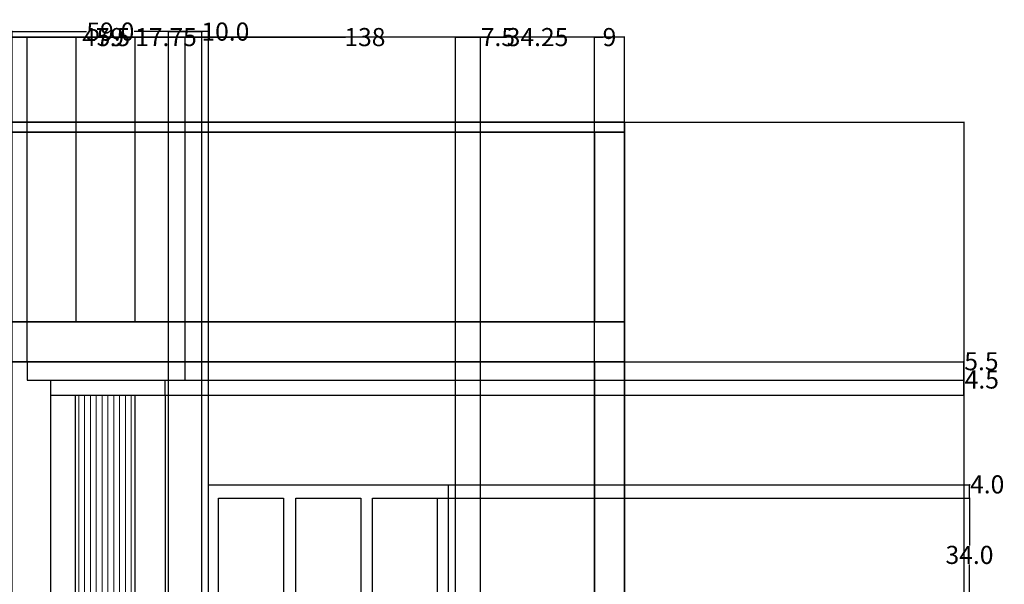
# Model space of a CAD drawing. Units: inches. Extents: x 12 to 590, y 127 to 569.
# Tile 4 of 4: x 294 to 590, y 399 to 569. Entities that reach past the tile are written whole.
import ezdxf

# ---------------------------------------------------------------- set-up
doc = ezdxf.new("R2010")
doc.units = ezdxf.units.IN
doc.header["$MEASUREMENT"] = 0
for name, color, linetype, lineweight in [('A-ANNO-DIMS', 2, 'Continuous', 18), ('A-COLS', 1, 'Continuous', 25), ('A-ELEV', 7, 'Continuous', 35), ('A-GLAZ', 4, 'Continuous', 25), ('A-WALL-PATT', 8, 'Continuous', 13)]:
    doc.layers.add(name, color=color, linetype=linetype, lineweight=lineweight)
doc.styles.get("Standard").update_dxf_attribs({"font": 'arial.ttf'})
doc.dimstyles.get("Standard").update_dxf_attribs({"dimtxt": 5.4375, "dimasz": 0.18, "dimexe": 0.18, "dimexo": 0.0625, "dimgap": 0.09, "dimtad": 0, "dimtih": 1, "dimtoh": 1, "dimdec": 4, "dimzin": 0, "dimdsep": 46, "dimlunit": 4, "dimtxsty": 'Standard', "dimcen": 0.09, "dimadec": 0, "dimazin": 0, "dimtfac": 1, "dimtdec": 4, "dimtofl": 0, "dimtmove": 0, "dimatfit": 3, "dimfxl": 1, "dimtolj": 1, "dimtzin": 0, "dimarcsym": 0})

# ---------------------------------------------------------------- blocks, each defined once
blk = doc.blocks.new('WIN-3PANE')
for points in [[(0, 41.5), (72, 41.5), (72, 0), (0, 0)], [(3, 37.5), (22.5, 37.5), (22.5, 3.5), (3, 3.5)], [(26.25, 37.5), (45.75, 37.5), (45.75, 3.5), (26.25, 3.5)], [(49.25, 37.5), (68.75, 37.5), (68.75, 3.5), (49.25, 3.5)]]:
    blk.add_lwpolyline(points, close=True)
blk = doc.blocks.new('*D7')
at = {"layer": 'A-ANNO-DIMS', "color": 0, "lineweight": -2, "transparency": 16777216}
for p, q in [((91.5, 538.06), (91.5, 563.73)), ((91.68, 563.55), (277.42, 563.55)), ((475.32, 563.55), (289.58, 563.55)), ((475.5, 538.06), (475.5, 563.73))]:
    blk.add_line(p, q, dxfattribs=at)
at = {"layer": 'A-ANNO-DIMS', "color": 0, "transparency": 16777216}
for points in [[(91.68, 563.58), (91.68, 563.52), (91.5, 563.55)], [(475.32, 563.58), (475.32, 563.52), (475.5, 563.55)]]:
    blk.add_solid(points, dxfattribs=at)
at = {"layer": 'Defpoints', "color": 0, "transparency": 16777216}
for p in [(475.5, 563.55), (91.5, 538), (475.5, 538)]:
    blk.add_point(p, dxfattribs=at)
at = {"layer": 'A-ANNO-DIMS', "color": 0, "transparency": 16777216, "insert": (283.5, 563.55), "char_height": 5.438, "attachment_point": 5}
blk.add_mtext('\\A1;384', dxfattribs=at)
blk = doc.blocks.new('*D8')
at = {"layer": 'A-ANNO-DIMS', "color": 0, "lineweight": -2, "transparency": 16777216}
for p, q in [((475.56, 538), (577.73, 538)), ((577.55, 537.82), (577.55, 350.53)), ((577.55, 157.5), (577.55, 344.79)), ((475.56, 157.32), (577.73, 157.32))]:
    blk.add_line(p, q, dxfattribs=at)
at = {"layer": 'A-ANNO-DIMS', "color": 0, "transparency": 16777216}
for points in [[(577.52, 537.82), (577.58, 537.82), (577.55, 538)], [(577.52, 157.5), (577.58, 157.5), (577.55, 157.32)]]:
    blk.add_solid(points, dxfattribs=at)
at = {"layer": 'Defpoints', "color": 0, "transparency": 16777216}
for p in [(475.5, 538), (475.5, 157.32), (577.55, 157.32)]:
    blk.add_point(p, dxfattribs=at)
at = {"layer": 'A-ANNO-DIMS', "color": 0, "transparency": 16777216, "insert": (577.55, 347.66), "char_height": 5.438, "attachment_point": 5}
blk.add_mtext('\\A1;380.7', dxfattribs=at)
blk = doc.blocks.new('*D11')
at = {"layer": 'A-ANNO-DIMS', "color": 0, "lineweight": -2, "transparency": 16777216}
for p, q in [((229.21, 535.06), (229.21, 563.73)), ((229.39, 563.55), (260.72, 563.55)), ((310.57, 563.55), (279.24, 563.55)), ((310.75, 535.06), (310.75, 563.73))]:
    blk.add_line(p, q, dxfattribs=at)
at = {"layer": 'A-ANNO-DIMS', "color": 0, "transparency": 16777216}
for points in [[(229.39, 563.58), (229.39, 563.52), (229.21, 563.55)], [(310.57, 563.58), (310.57, 563.52), (310.75, 563.55)]]:
    blk.add_solid(points, dxfattribs=at)
at = {"layer": 'Defpoints', "color": 0, "transparency": 16777216}
for p in [(310.75, 563.55), (229.21, 535), (310.75, 535)]:
    blk.add_point(p, dxfattribs=at)
at = {"layer": 'A-ANNO-DIMS', "color": 0, "transparency": 16777216, "insert": (269.98, 563.55), "char_height": 5.438, "attachment_point": 5}
blk.add_mtext('\\A1;81.54', dxfattribs=at)
blk = doc.blocks.new('*D12')
at = {"layer": 'A-ANNO-DIMS', "color": 0, "lineweight": -2, "transparency": 16777216}
for p, q in [((310.75, 535.06), (310.75, 563.73)), ((310.93, 563.55), (328.32, 563.55)), ((328.5, 535.06), (328.5, 563.73)), ((328.5, 563.55), (328.68, 563.55))]:
    blk.add_line(p, q, dxfattribs=at)
at = {"layer": 'A-ANNO-DIMS', "color": 0, "transparency": 16777216}
for points in [[(310.93, 563.58), (310.93, 563.52), (310.75, 563.55)], [(328.32, 563.58), (328.32, 563.52), (328.5, 563.55)]]:
    blk.add_solid(points, dxfattribs=at)
at = {"layer": 'Defpoints', "color": 0, "transparency": 16777216}
for p in [(328.5, 563.55), (310.75, 535), (328.5, 535)]:
    blk.add_point(p, dxfattribs=at)
at = {"layer": 'A-ANNO-DIMS', "color": 0, "transparency": 16777216, "insert": (337.71, 563.55), "char_height": 5.438, "attachment_point": 5}
blk.add_mtext('\\A1;17.75', dxfattribs=at)
blk = doc.blocks.new('*D13')
at = {"layer": 'A-ANNO-DIMS', "color": 0, "lineweight": -2, "transparency": 16777216}
for p, q in [((328.5, 535.06), (328.5, 563.73)), ((328.68, 563.55), (391.65, 563.55)), ((466.32, 563.55), (403.35, 563.55)), ((466.5, 535.06), (466.5, 563.73))]:
    blk.add_line(p, q, dxfattribs=at)
at = {"layer": 'A-ANNO-DIMS', "color": 0, "transparency": 16777216}
for points in [[(328.68, 563.58), (328.68, 563.52), (328.5, 563.55)], [(466.32, 563.58), (466.32, 563.52), (466.5, 563.55)]]:
    blk.add_solid(points, dxfattribs=at)
at = {"layer": 'Defpoints', "color": 0, "transparency": 16777216}
for p in [(466.5, 563.55), (328.5, 535), (466.5, 535)]:
    blk.add_point(p, dxfattribs=at)
at = {"layer": 'A-ANNO-DIMS', "color": 0, "transparency": 16777216, "insert": (397.5, 563.55), "char_height": 5.438, "attachment_point": 5}
blk.add_mtext('\\A1;138', dxfattribs=at)
blk = doc.blocks.new('*D14')
at = {"layer": 'A-ANNO-DIMS', "color": 0, "lineweight": -2, "transparency": 16777216}
for p, q in [((466.5, 535.06), (466.5, 563.73)), ((466.68, 563.55), (469.12, 563.55)), ((475.32, 563.55), (472.88, 563.55)), ((475.5, 535.06), (475.5, 563.73))]:
    blk.add_line(p, q, dxfattribs=at)
at = {"layer": 'A-ANNO-DIMS', "color": 0, "transparency": 16777216}
for points in [[(466.68, 563.58), (466.68, 563.52), (466.5, 563.55)], [(475.32, 563.58), (475.32, 563.52), (475.5, 563.55)]]:
    blk.add_solid(points, dxfattribs=at)
at = {"layer": 'Defpoints', "color": 0, "transparency": 16777216}
for p in [(475.5, 563.55), (466.5, 535), (475.5, 535)]:
    blk.add_point(p, dxfattribs=at)
at = {"layer": 'A-ANNO-DIMS', "color": 0, "transparency": 16777216, "insert": (471, 563.55), "char_height": 5.438, "attachment_point": 5}
blk.add_mtext('\\A1;9', dxfattribs=at)
blk = doc.blocks.new('*D28')
at = {"layer": 'A-ANNO-DIMS', "color": 0, "lineweight": -2, "transparency": 16777216}
for p, q in [((291.5, 429.06), (291.5, 563.73)), ((291.68, 563.55), (317.01, 563.55)), ((350.32, 563.55), (324.99, 563.55)), ((350.5, 429.06), (350.5, 563.73))]:
    blk.add_line(p, q, dxfattribs=at)
at = {"layer": 'A-ANNO-DIMS', "color": 0, "transparency": 16777216}
for points in [[(291.68, 563.58), (291.68, 563.52), (291.5, 563.55)], [(350.32, 563.58), (350.32, 563.52), (350.5, 563.55)]]:
    blk.add_solid(points, dxfattribs=at)
at = {"layer": 'Defpoints', "color": 0, "transparency": 16777216}
for p in [(350.5, 563.55), (291.5, 429), (350.5, 429)]:
    blk.add_point(p, dxfattribs=at)
at = {"layer": 'A-ANNO-DIMS', "color": 0, "transparency": 16777216, "insert": (321, 563.55), "char_height": 5.438, "attachment_point": 5}
blk.add_mtext('\\A1;59', dxfattribs=at)
blk = doc.blocks.new('*D39')
at = {"layer": 'A-ANNO-DIMS', "color": 0, "lineweight": -2, "transparency": 16777216}
for p, q in [((296, 466.06), (296, 563.73)), ((296.18, 563.55), (312.47, 563.55)), ((343.32, 563.55), (327.03, 563.55)), ((343.5, 466.06), (343.5, 563.73))]:
    blk.add_line(p, q, dxfattribs=at)
at = {"layer": 'A-ANNO-DIMS', "color": 0, "transparency": 16777216}
for points in [[(296.18, 563.58), (296.18, 563.52), (296, 563.55)], [(343.32, 563.58), (343.32, 563.52), (343.5, 563.55)]]:
    blk.add_solid(points, dxfattribs=at)
at = {"layer": 'Defpoints', "color": 0, "transparency": 16777216}
for p in [(343.5, 563.55), (296, 466), (343.5, 466)]:
    blk.add_point(p, dxfattribs=at)
at = {"layer": 'A-ANNO-DIMS', "color": 0, "transparency": 16777216, "insert": (319.75, 563.55), "char_height": 5.438, "attachment_point": 5}
blk.add_mtext('\\A1;47.5', dxfattribs=at)
blk = doc.blocks.new('*D40')
at = {"layer": 'A-ANNO-DIMS', "color": 0, "lineweight": -2, "transparency": 16777216}
for p, q in [((303, 455.94), (303, 131.59)), ((337.5, 455.94), (337.5, 131.59)), ((303.18, 131.77), (313.08, 131.77)), ((337.32, 131.77), (327.42, 131.77))]:
    blk.add_line(p, q, dxfattribs=at)
at = {"layer": 'A-ANNO-DIMS', "color": 0, "transparency": 16777216}
for points in [[(303.18, 131.8), (303.18, 131.74), (303, 131.77)], [(337.32, 131.8), (337.32, 131.74), (337.5, 131.77)]]:
    blk.add_solid(points, dxfattribs=at)
at = {"layer": 'Defpoints', "color": 0, "transparency": 16777216}
for p in [(303, 456), (337.5, 456), (337.5, 131.77)]:
    blk.add_point(p, dxfattribs=at)
at = {"layer": 'A-ANNO-DIMS', "color": 0, "transparency": 16777216, "insert": (320.25, 131.77), "char_height": 5.438, "attachment_point": 5}
blk.add_mtext('\\A1;34.5', dxfattribs=at)
blk = doc.blocks.new('*D41')
at = {"layer": 'A-ANNO-DIMS', "color": 0, "lineweight": -2, "transparency": 16777216}
for p, q in [((343.56, 466), (577.73, 466)), ((577.55, 466), (577.55, 466.18)), ((577.55, 466.18), (577.73, 466.18)), ((577.55, 460.68), (577.55, 465.82)), ((343.56, 460.5), (577.73, 460.5))]:
    blk.add_line(p, q, dxfattribs=at)
at = {"layer": 'A-ANNO-DIMS', "color": 0, "transparency": 16777216}
for points in [[(577.52, 465.82), (577.58, 465.82), (577.55, 466)], [(577.52, 460.68), (577.58, 460.68), (577.55, 460.5)]]:
    blk.add_solid(points, dxfattribs=at)
at = {"layer": 'Defpoints', "color": 0, "transparency": 16777216}
for p in [(343.5, 466), (577.55, 466), (343.5, 460.5)]:
    blk.add_point(p, dxfattribs=at)
at = {"layer": 'A-ANNO-DIMS', "color": 0, "transparency": 16777216, "insert": (582.79, 466.18), "char_height": 5.438, "attachment_point": 5}
blk.add_mtext('\\A1;5.5', dxfattribs=at)
blk = doc.blocks.new('*D42')
at = {"layer": 'A-ANNO-DIMS', "color": 0, "lineweight": -2, "transparency": 16777216}
for p, q in [((337.56, 460.5), (577.73, 460.5)), ((577.55, 460.5), (577.55, 460.68)), ((577.55, 460.68), (577.73, 460.68)), ((577.55, 456.18), (577.55, 460.32)), ((337.56, 456), (577.73, 456))]:
    blk.add_line(p, q, dxfattribs=at)
at = {"layer": 'A-ANNO-DIMS', "color": 0, "transparency": 16777216}
for points in [[(577.52, 460.32), (577.58, 460.32), (577.55, 460.5)], [(577.52, 456.18), (577.58, 456.18), (577.55, 456)]]:
    blk.add_solid(points, dxfattribs=at)
at = {"layer": 'Defpoints', "color": 0, "transparency": 16777216}
for p in [(337.5, 460.5), (577.55, 460.5), (337.5, 456)]:
    blk.add_point(p, dxfattribs=at)
at = {"layer": 'A-ANNO-DIMS', "color": 0, "transparency": 16777216, "insert": (582.9, 460.68), "char_height": 5.438, "attachment_point": 5}
blk.add_mtext('\\A1;4.5', dxfattribs=at)
blk = doc.blocks.new('*D49')
at = {"layer": 'A-ANNO-DIMS', "color": 0, "lineweight": -2, "transparency": 16777216}
for p, q in [((424.75, 374.06), (424.75, 563.73)), ((424.93, 563.55), (432.07, 563.55)), ((432.25, 376.06), (432.25, 563.73)), ((432.25, 563.55), (432.43, 563.55))]:
    blk.add_line(p, q, dxfattribs=at)
at = {"layer": 'A-ANNO-DIMS', "color": 0, "transparency": 16777216}
for points in [[(424.93, 563.58), (424.93, 563.52), (424.75, 563.55)], [(432.07, 563.58), (432.07, 563.52), (432.25, 563.55)]]:
    blk.add_solid(points, dxfattribs=at)
at = {"layer": 'Defpoints', "color": 0, "transparency": 16777216}
for p in [(432.25, 563.55), (432.25, 376), (424.75, 374)]:
    blk.add_point(p, dxfattribs=at)
at = {"layer": 'A-ANNO-DIMS', "color": 0, "transparency": 16777216, "insert": (437.47, 563.55), "char_height": 5.438, "attachment_point": 5}
blk.add_mtext('\\A1;7.5', dxfattribs=at)
blk = doc.blocks.new('*D50')
at = {"layer": 'A-ANNO-DIMS', "color": 0, "lineweight": -2, "transparency": 16777216}
for p, q in [((432.25, 376.06), (432.25, 563.73)), ((432.43, 563.55), (440.09, 563.55)), ((466.32, 563.55), (458.66, 563.55)), ((466.5, 376.06), (466.5, 563.73))]:
    blk.add_line(p, q, dxfattribs=at)
at = {"layer": 'A-ANNO-DIMS', "color": 0, "transparency": 16777216}
for points in [[(432.43, 563.58), (432.43, 563.52), (432.25, 563.55)], [(466.32, 563.58), (466.32, 563.52), (466.5, 563.55)]]:
    blk.add_solid(points, dxfattribs=at)
at = {"layer": 'Defpoints', "color": 0, "transparency": 16777216}
for p in [(466.5, 563.55), (432.25, 376), (466.5, 376)]:
    blk.add_point(p, dxfattribs=at)
at = {"layer": 'A-ANNO-DIMS', "color": 0, "transparency": 16777216, "insert": (449.38, 563.55), "char_height": 5.438, "attachment_point": 5}
blk.add_mtext('\\A1;34.25', dxfattribs=at)
blk = doc.blocks.new('*D60')
at = {"layer": 'A-ANNO-DIMS', "color": 0, "lineweight": -2, "transparency": 16777216}
for p, q in [((291.5, 285.06), (291.5, 565.38)), ((350.5, 285.06), (350.5, 565.38)), ((291.68, 565.2), (313.86, 565.2)), ((350.32, 565.2), (328.14, 565.2))]:
    blk.add_line(p, q, dxfattribs=at)
at = {"layer": 'A-ANNO-DIMS', "color": 0, "transparency": 16777216}
for points in [[(291.68, 565.23), (291.68, 565.17), (291.5, 565.2)], [(350.32, 565.23), (350.32, 565.17), (350.5, 565.2)]]:
    blk.add_solid(points, dxfattribs=at)
at = {"layer": 'Defpoints', "color": 0, "transparency": 16777216}
for p in [(350.5, 565.2), (291.5, 285), (350.5, 285)]:
    blk.add_point(p, dxfattribs=at)
at = {"layer": 'A-ANNO-DIMS', "color": 0, "transparency": 16777216, "insert": (321, 565.2), "char_height": 5.438, "attachment_point": 5}
blk.add_mtext('\\A1;59.0', dxfattribs=at)
blk = doc.blocks.new('*D62')
at = {"layer": 'A-ANNO-DIMS', "color": 0, "lineweight": -2, "transparency": 16777216}
for p, q in [((338.5, 181.5625), (338.5, 565.38)), ((348.5, 181.5625), (348.5, 565.38)), ((338.68, 565.2), (348.32, 565.2)), ((348.5, 565.2), (348.68, 565.2))]:
    blk.add_line(p, q, dxfattribs=at)
at = {"layer": 'A-ANNO-DIMS', "color": 0, "transparency": 16777216}
for points in [[(338.68, 565.23), (338.68, 565.17), (338.5, 565.2)], [(348.32, 565.23), (348.32, 565.17), (348.5, 565.2)]]:
    blk.add_solid(points, dxfattribs=at)
at = {"layer": 'Defpoints', "color": 0, "transparency": 16777216}
for p in [(348.5, 565.2), (338.5, 181.5), (348.5, 181.5)]:
    blk.add_point(p, dxfattribs=at)
at = {"layer": 'A-ANNO-DIMS', "color": 0, "transparency": 16777216, "insert": (355.566875, 565.2), "char_height": 5.4375, "attachment_point": 5}
blk.add_mtext('\\A1;10.0', dxfattribs=at)
blk = doc.blocks.new('*D72')
at = {"layer": 'A-ANNO-DIMS', "color": 0, "lineweight": -2, "transparency": 16777216}
for p, q in [((419.31, 425), (579.38, 425)), ((579.2, 424.82), (579.2, 410.87)), ((579.2, 391.18), (579.2, 405.13)), ((419.31, 391), (579.38, 391))]:
    blk.add_line(p, q, dxfattribs=at)
at = {"layer": 'A-ANNO-DIMS', "color": 0, "transparency": 16777216}
for points in [[(579.17, 424.82), (579.23, 424.82), (579.2, 425)], [(579.17, 391.18), (579.23, 391.18), (579.2, 391)]]:
    blk.add_solid(points, dxfattribs=at)
at = {"layer": 'Defpoints', "color": 0, "transparency": 16777216}
for p in [(419.25, 425), (579.2, 425), (419.25, 391)]:
    blk.add_point(p, dxfattribs=at)
at = {"layer": 'A-ANNO-DIMS', "color": 0, "transparency": 16777216, "insert": (579.2, 408), "char_height": 5.438, "attachment_point": 5}
blk.add_mtext('\\A1;34.0', dxfattribs=at)
blk = doc.blocks.new('*D73')
at = {"layer": 'A-ANNO-DIMS', "color": 0, "lineweight": -2, "transparency": 16777216}
for p, q in [((579.2, 429), (579.2, 429.18)), ((579.2, 429.18), (579.38, 429.18)), ((422.56, 429), (579.38, 429)), ((579.2, 425.18), (579.2, 428.82)), ((419.31, 425), (579.38, 425))]:
    blk.add_line(p, q, dxfattribs=at)
at = {"layer": 'A-ANNO-DIMS', "color": 0, "transparency": 16777216}
for points in [[(579.17, 428.82), (579.23, 428.82), (579.2, 429)], [(579.17, 425.18), (579.23, 425.18), (579.2, 425)]]:
    blk.add_solid(points, dxfattribs=at)
at = {"layer": 'Defpoints', "color": 0, "transparency": 16777216}
for p in [(422.5, 429), (579.2, 429), (419.25, 425)]:
    blk.add_point(p, dxfattribs=at)
at = {"layer": 'A-ANNO-DIMS', "color": 0, "transparency": 16777216, "insert": (584.52, 429.18), "char_height": 5.438, "attachment_point": 5}
blk.add_mtext('\\A1;4.0', dxfattribs=at)

msp = doc.modelspace()

# ---------------------------------------------------------------- hatches: boundary and pattern name
at = {"layer": 'A-WALL-PATT'}
h = msp.add_hatch(dxfattribs=at)
h.set_pattern_fill('ANSI31', color=256, scale=14, angle=45)
h.paths.add_polyline_path([(328.5, 456), (310.5, 456), (310.5, 379.5), (310.5, 376), (328.5, 376)])
h.paths.add_polyline_path([(328.5, 322), (310.5, 322), (310.5, 193.5), (328.5, 193.5)])

# ---------------------------------------------------------------- linework, layer by layer
at = {"layer": 'A-COLS'}
for p, q in [((310.75, 478), (310.75, 535)), ((328.5, 478), (328.5, 535)), ((296, 466), (296, 460.5)), ((343.5, 460.5), (343.5, 466)), ((296, 460.5), (343.5, 460.5)), ((303, 460.5), (303, 456)), ((337.5, 456), (337.5, 460.5)), ((303, 456), (337.5, 456)), ((310.5, 379.5), (310.5, 456)), ((328.5, 376), (328.5, 456))]:
    msp.add_line(p, q, dxfattribs=at)
at = {"layer": 'A-ELEV'}
for p, q in [((475.5, 538), (91.5, 538)), ((475.5, 535), (475.5, 538)), ((102, 535), (466.5, 535)), ((466.5, 535), (466.5, 478)), ((475.5, 535), (466.5, 535)), ((475.5, 484.5), (475.5, 535)), ((475.5, 322), (475.5, 484.5)), ((146, 478), (475.5, 478)), ((122, 466), (451.5, 466)), ((466.5, 466), (451.5, 466)), ((466.5, 322), (466.5, 466)), ((466.5, 466), (475.5, 466))]:
    msp.add_line(p, q, dxfattribs=at)

# ---------------------------------------------------------------- block references
at = {"layer": 'A-GLAZ'}
msp.add_blockref('WIN-3PANE', (350.5, 387.5), dxfattribs=at)

# ---------------------------------------------------------------- dimensions: what is measured, and where the dimension line sits
at = {"layer": 'A-ANNO-DIMS'}
for base, p1, p2, override, picture, middle in [((350.5, 565.2), (291.5, 285), (350.5, 285), {"dimdec": 1, "dimlfac": 1, "dimrnd": 0, "dimzin": 0, "dimdsep": 46, "dimlunit": 2}, '*D60', (321, 565.2)), ((348.5, 565.2), (338.5, 181.5), (348.5, 181.5), {"dimdec": 1, "dimlfac": 1, "dimrnd": 0, "dimzin": 0, "dimdsep": 46, "dimlunit": 2}, '*D62', (355.5669, 565.2)), ((475.5, 563.55), (91.5, 538), (475.5, 538), {"dimdec": 0, "dimlfac": 1, "dimrnd": 0, "dimzin": 0, "dimdsep": 46, "dimlunit": 2}, '*D7', (283.5, 563.55)), ((310.75, 563.55), (229.2101, 535), (310.75, 535), {"dimdec": 2, "dimlfac": 1, "dimrnd": 0, "dimzin": 0, "dimdsep": 46, "dimlunit": 2}, '*D11', (269.9801, 563.55)), ((350.5, 563.55), (291.5, 429), (350.5, 429), {"dimdec": 0, "dimlfac": 1, "dimrnd": 0, "dimzin": 0, "dimdsep": 46, "dimlunit": 2}, '*D28', (321, 563.55)), ((343.5, 563.55), (296, 466), (343.5, 466), {"dimdec": 1, "dimlfac": 1, "dimrnd": 0, "dimzin": 0, "dimdsep": 46, "dimlunit": 2}, '*D39', (319.75, 563.55)), ((328.5, 563.55), (310.75, 535), (328.5, 535), {"dimdec": 2, "dimlfac": 1, "dimrnd": 0, "dimzin": 0, "dimdsep": 46, "dimlunit": 2}, '*D12', (337.7089, 563.55)), ((466.5, 563.55), (328.5, 535), (466.5, 535), {"dimdec": 0, "dimlfac": 1, "dimrnd": 0, "dimzin": 0, "dimdsep": 46, "dimlunit": 2}, '*D13', (397.5, 563.55)), ((432.25, 563.55), (424.75, 374), (432.25, 376), {"dimdec": 1, "dimlfac": 1, "dimrnd": 0, "dimzin": 0, "dimdsep": 46, "dimlunit": 2}, '*D49', (437.4679, 563.55)), ((466.5, 563.55), (432.25, 376), (466.5, 376), {"dimdec": 2, "dimlfac": 1, "dimrnd": 0, "dimzin": 0, "dimdsep": 46, "dimlunit": 2}, '*D50', (449.375, 563.55)), ((475.5, 563.55), (466.5, 535), (475.5, 535), {"dimdec": 0, "dimlfac": 1, "dimrnd": 0, "dimzin": 0, "dimdsep": 46, "dimlunit": 2}, '*D14', (471, 563.55)), ((337.5, 131.7663), (303, 456), (337.5, 456), {"dimdec": 1, "dimlfac": 1, "dimrnd": 0, "dimzin": 0, "dimdsep": 46, "dimlunit": 2}, '*D40', (320.25, 131.7663))]:
    dim = msp.add_linear_dim(base=base, p1=p1, p2=p2, dimstyle='Standard', override=override, dxfattribs=at)
    dim.commit()
    dim.dimension.update_dxf_attribs({"geometry": picture, "text_midpoint": middle})
for base, p1, p2, picture, middle in [((577.55, 157.3163), (475.5, 538), (475.5, 157.3163), '*D8', (577.55, 347.6581)), ((577.55, 466), (343.5, 460.5), (343.5, 466), '*D41', (582.7902, 466.18)), ((577.55, 460.5), (337.5, 456), (337.5, 460.5), '*D42', (582.8996, 460.68)), ((579.2, 429), (419.25, 425), (422.5, 429), '*D73', (584.5199, 429.18)), ((579.2, 425), (419.25, 391), (419.25, 425), '*D72', (579.2, 408))]:
    dim = msp.add_linear_dim(base=base, p1=p1, p2=p2, angle=90, dimstyle='Standard', override={"dimdec": 1, "dimlfac": 1, "dimrnd": 0, "dimzin": 0, "dimdsep": 46, "dimlunit": 2}, dxfattribs=at)
    dim.commit()
    dim.dimension.update_dxf_attribs({"geometry": picture, "text_midpoint": middle})

doc.saveas('drawing.dxf')
